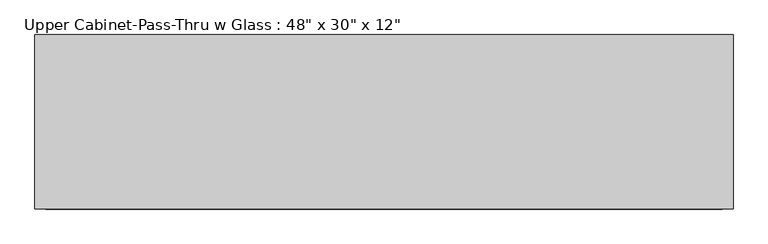
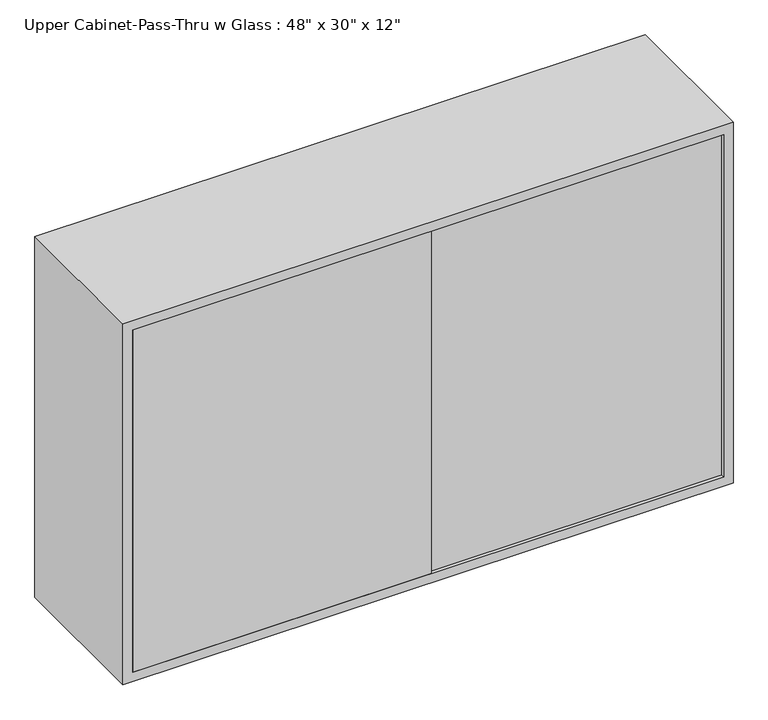
"""IFC4 building model written with IfcOpenShell, lengths in millimetres: furniture geometry."""

from ifc_helpers import new_model, si_unit, frame, origin, place, context, project, spatial, polyline, outline, extrude, source, transform, mapped, element, save


def furniture_f491f192(model_context):
    return source(origin(), model_context, "Body", "SweptSolid", [
        extrude(outline(polyline([(1371.6, 628.3377049), (2133.6, 628.3377049), (2133.6, -590.8622951), (1371.6, -590.8622951), (1371.6, 628.3377049)]), holes=[polyline([(1390.65, 609.2877049), (1390.65, -571.8122951), (2114.55, -571.8122951), (2114.55, 609.2877049), (1390.65, 609.2877049)])]), frame((0.0, -304.8, 0.0), z_axis=(0.0, 1.0, 0.0), x_axis=(0.0, 0.0, 1.0)), (0.0, 0.0, 1.0), 304.8),
        extrude(outline(polyline([(25.0877049, -304.8), (-571.8122951, -304.8), (-571.8122951, -298.45), (25.0877049, -298.45), (25.0877049, -304.8)])), frame((0.0, 0.0, 1390.65), z_axis=(0.0, 0.0, 1.0), x_axis=(1.0, 0.0, 0.0)), (0.0, 0.0, 1.0), 723.9),
        extrude(outline(polyline([(609.2877049, -6.35), (12.3877049, -6.35), (12.3877049, 0.0), (609.2877049, 0.0), (609.2877049, -6.35)])), frame((0.0, 0.0, 1390.65), z_axis=(0.0, 0.0, 1.0), x_axis=(1.0, 0.0, 0.0)), (0.0, 0.0, 1.0), 723.9),
        extrude(outline(polyline([(609.2877049, -298.45), (12.3877049, -298.45), (12.3877049, -292.1), (609.2877049, -292.1), (609.2877049, -298.45)])), frame((0.0, 0.0, 1390.65), z_axis=(0.0, 0.0, 1.0), x_axis=(1.0, 0.0, 0.0)), (0.0, 0.0, 1.0), 723.9),
        extrude(outline(polyline([(25.0877049, -12.7), (-571.8122951, -12.7), (-571.8122951, -6.35), (25.0877049, -6.35), (25.0877049, -12.7)])), frame((0.0, 0.0, 1390.65), z_axis=(0.0, 0.0, 1.0), x_axis=(1.0, 0.0, 0.0)), (0.0, 0.0, 1.0), 723.9),
        extrude(outline(polyline([(609.2877049, -285.75), (-571.8122951, -285.75), (-571.8122951, -19.05), (609.2877049, -19.05), (609.2877049, -285.75)])), frame((0.0, 0.0, 1873.25), z_axis=(0.0, 0.0, 1.0), x_axis=(1.0, 0.0, 0.0)), (0.0, 0.0, 1.0), 12.7),
        extrude(outline(polyline([(609.2877049, -285.75), (-571.8122951, -285.75), (-571.8122951, -19.05), (609.2877049, -19.05), (609.2877049, -285.75)])), frame((0.0, 0.0, 1619.25), z_axis=(0.0, 0.0, 1.0), x_axis=(1.0, 0.0, 0.0)), (0.0, 0.0, 1.0), 12.7),
    ])


if __name__ == "__main__":
    model = new_model("IFC4")
    model_context = context("Model", 3, world=origin())
    ifc_project = project(units=[si_unit("LENGTHUNIT", "METRE", prefix="MILLI")], contexts=[model_context])
    site = spatial("IfcSite", under=ifc_project)
    building = spatial("IfcBuilding", under=site)
    placement = place(None, origin())
    furniture_shape = furniture_f491f192(model_context)
    element("IfcFurniture", 1, ObjectType="Upper Cabinet-Pass-Thru w Glass : 48\" x 30\" x 12\"", at=placement, inside=building, context=model_context, shape_type="MappedRepresentation", body=[
        mapped(furniture_shape, transform((0.0, 0.0, 0.0), x_axis=(1.0, 0.0, 0.0), y_axis=(0.0, 1.0, 0.0), z_axis=(0.0, 0.0, 1.0))),
    ])
    save(model, "model.ifc")

# Revit data of these elements
# Type "Upper Cabinet-Pass-Thru w Glass : 48\" x 30\" x 12\""
#   Depth = 1' - 0"
#   Height = 2' - 6"
#   Top Of Cabinet = 7' - 0"
#   Width = 4' - 0"
#   Default Elevation = 0
# Element 1 (IfcFurniture, "Upper Cabinet-Pass-Thru w Glass : 48\" x 30\" x 12\"")
#   Materials on its faces: "Glass", "Cabinet"
# Materials
#   "Glass": class "Glass", colour RGB 0 128 192, transparency 0.75, Description = "Soda Lime Glass", Cost = 0
#   "Cabinet": colour RGB 204 122 2, transparency 0
